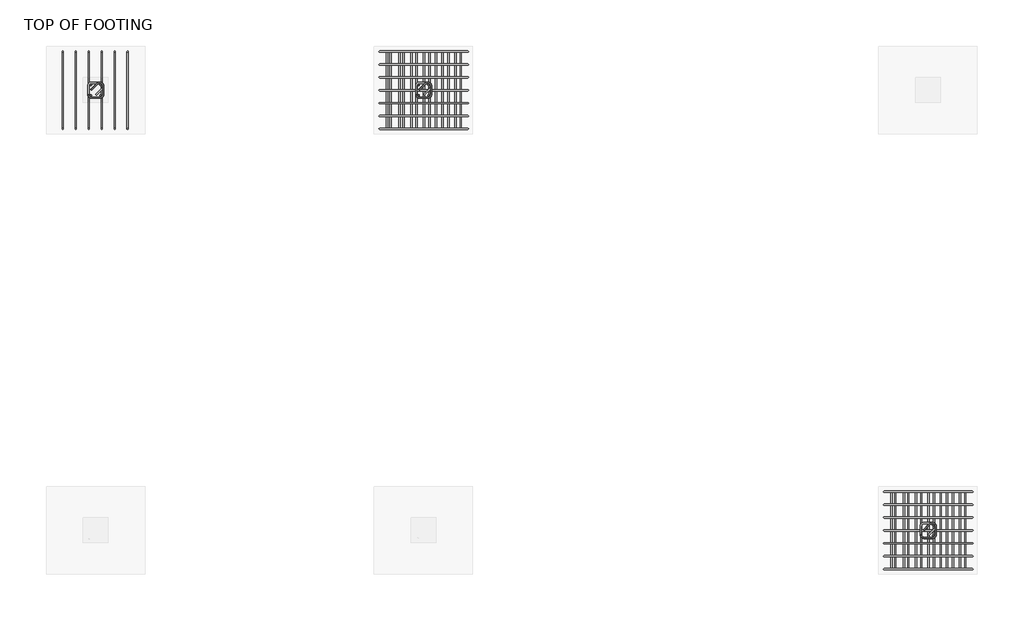
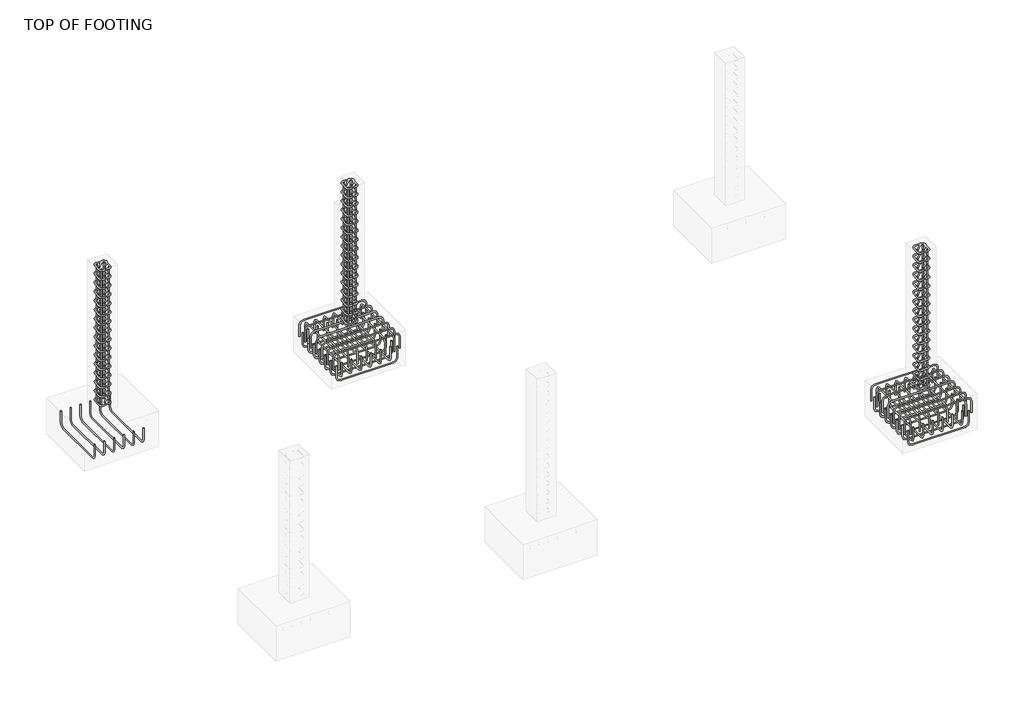
# One storey, part 3 of 6: 17 reinforcing bars.
"""IFC4 building model written with IfcOpenShell, lengths in millimetres."""

from ifc_helpers import new_model, si_unit, point, frame, origin, place, context, project, spatial, polyline, circle_curve, trimmed, segment, composite_curve, source, transform, mapped, element, save
from ifc_brep_helpers import swept_disk

model = new_model("IFC4")

# Units and contexts
model_context = context("Model", 3, world=origin())
ifc_project = project(units=[si_unit("LENGTHUNIT", "METRE", prefix="MILLI")], contexts=[model_context])

# Site, building, storey
site = spatial("IfcSite", under=ifc_project)
building = spatial("IfcBuilding", under=site)
storey = spatial("IfcBuildingStorey", under=building, Name="TOP OF FOOTING", Elevation=-1828.8)

# Reinforcing bars
placement = place(None, origin())
reinforcing_bar_shape = source(origin(), model_context, "Body", "SolidModel", [
    swept_disk(composite_curve([segment(polyline([(-15225.2448384, 120.9474721, -2014.7438142), (-15225.2448384, 120.9474721, -2162.0438142)]), True, "CONTINUOUS"), segment(trimmed(circle_curve(frame((-15225.2448384, 74.5974721, -2162.0438142), z_axis=(-1.0, 0.0, 0.0), x_axis=(0.0, 46.349999999999994, 0.0)), 46.35), [point((-15225.2448384, 120.9474721, -2162.0438142))], [point((-15225.2448384, 74.5974721, -2208.3938142))], True, "CARTESIAN"), True, "CONTINUOUS"), segment(polyline([(-15225.2448384, 74.5974721, -2208.3938142), (-15225.2448384, -540.0025279, -2208.3938142)]), True, "CONTINUOUS"), segment(trimmed(circle_curve(frame((-15225.2448384, -540.0025279, -2162.0438142), z_axis=(-1.0, 0.0, 0.0), x_axis=(0.0, 0.0, -46.350000000000364)), 46.35), [point((-15225.2448384, -540.0025279, -2208.3938142))], [point((-15225.2448384, -586.3525279, -2162.0438142))], True, "CARTESIAN"), True, "CONTINUOUS"), segment(polyline([(-15225.2448384, -586.3525279, -2162.0438142), (-15225.2448384, -586.3525279, -2014.7438142)]), True, "CONTINUOUS")], self_intersect=False), 6.35),
])
element("IfcReinforcingBar", 1, at=placement, inside=storey, context=model_context, shape_type="MappedRepresentation", body=[
    mapped(reinforcing_bar_shape, transform((0.0, 0.0, 0.0), x_axis=(1.0, 0.0, 0.0), y_axis=(0.0, 1.0, 0.0), z_axis=(0.0, 0.0, 1.0))),
    mapped(reinforcing_bar_shape, transform((118.647936, 0.0, 0.0), x_axis=(1.0, 0.0, 0.0), y_axis=(0.0, 1.0, 0.0), z_axis=(0.0, 0.0, 1.0))),
    mapped(reinforcing_bar_shape, transform((237.295872, 0.0, 0.0), x_axis=(1.0, 0.0, 0.0), y_axis=(0.0, 1.0, 0.0), z_axis=(0.0, 0.0, 1.0))),
    mapped(reinforcing_bar_shape, transform((355.943808, 0.0, 0.0), x_axis=(1.0, 0.0, 0.0), y_axis=(0.0, 1.0, 0.0), z_axis=(0.0, 0.0, 1.0))),
    mapped(reinforcing_bar_shape, transform((474.591744, 0.0, 0.0), x_axis=(1.0, 0.0, 0.0), y_axis=(0.0, 1.0, 0.0), z_axis=(0.0, 0.0, 1.0))),
    mapped(reinforcing_bar_shape, transform((593.23968, 0.0, 0.0), x_axis=(1.0, 0.0, 0.0), y_axis=(0.0, 1.0, 0.0), z_axis=(0.0, 0.0, 1.0))),
])
reinforcing_bar_2_shape = source(origin(), model_context, "Body", "SolidModel", [
    swept_disk(composite_curve([segment(polyline([(-11554.9855212, 120.9474721, -2038.8), (-11554.9855212, 120.9474721, -2186.1)]), True, "CONTINUOUS"), segment(trimmed(circle_curve(frame((-11601.3355212, 120.9474721, -2186.1), z_axis=(0.0, 1.0, 0.0), x_axis=(46.350000000000364, 0.0, 0.0)), 46.35), [point((-11554.9855212, 120.9474721, -2186.1))], [point((-11601.3355212, 120.9474721, -2232.45))], True, "CARTESIAN"), True, "CONTINUOUS"), segment(polyline([(-11601.3355212, 120.9474721, -2232.45), (-12244.4761323, 120.9474721, -2232.45)]), True, "CONTINUOUS"), segment(trimmed(circle_curve(frame((-12244.4761323, 120.9474721, -2186.1), z_axis=(0.0, 1.0, 0.0), x_axis=(0.0, 0.0, -46.34999999999991)), 46.35), [point((-12244.4761323, 120.9474721, -2232.45))], [point((-12290.8261323, 120.9474721, -2186.1))], True, "CARTESIAN"), True, "CONTINUOUS"), segment(polyline([(-12290.8261323, 120.9474721, -2186.1), (-12290.8261323, 120.9474721, -2038.8)]), True, "CONTINUOUS")], self_intersect=False), 6.35),
])
element("IfcReinforcingBar", 2, at=placement, inside=storey, context=model_context, shape_type="MappedRepresentation", body=[
    mapped(reinforcing_bar_2_shape, transform((0.0, 0.0, 0.0), x_axis=(1.0, 0.0, 0.0), y_axis=(0.0, 1.0, 0.0), z_axis=(0.0, 0.0, 1.0))),
    mapped(reinforcing_bar_2_shape, transform((0.0, -117.8833333, 0.0), x_axis=(1.0, 0.0, 0.0), y_axis=(0.0, 1.0, 0.0), z_axis=(0.0, 0.0, 1.0))),
    mapped(reinforcing_bar_2_shape, transform((0.0, -235.7666667, 0.0), x_axis=(1.0, 0.0, 0.0), y_axis=(0.0, 1.0, 0.0), z_axis=(0.0, 0.0, 1.0))),
    mapped(reinforcing_bar_2_shape, transform((0.0, -353.65, 0.0), x_axis=(1.0, 0.0, 0.0), y_axis=(0.0, 1.0, 0.0), z_axis=(0.0, 0.0, 1.0))),
    mapped(reinforcing_bar_2_shape, transform((0.0, -471.5333333, 0.0), x_axis=(1.0, 0.0, 0.0), y_axis=(0.0, 1.0, 0.0), z_axis=(0.0, 0.0, 1.0))),
    mapped(reinforcing_bar_2_shape, transform((0.0, -589.4166667, 0.0), x_axis=(1.0, 0.0, 0.0), y_axis=(0.0, 1.0, 0.0), z_axis=(0.0, 0.0, 1.0))),
    mapped(reinforcing_bar_2_shape, transform((0.0, -707.3, 0.0), x_axis=(1.0, 0.0, 0.0), y_axis=(0.0, 1.0, 0.0), z_axis=(0.0, 0.0, 1.0))),
])
reinforcing_bar_3_shape = source(origin(), model_context, "Body", "SolidModel", [
    swept_disk(composite_curve([segment(polyline([(-12330.2056799, 120.9474721, -2070.9463075), (-12330.2056799, 120.9474721, -1923.6463075)]), True, "CONTINUOUS"), segment(trimmed(circle_curve(frame((-12283.8556799, 120.9474721, -1923.6463075), z_axis=(0.0, 1.0, 0.0), x_axis=(-46.350000000000364, 0.0, 0.0)), 46.35), [point((-12330.2056799, 120.9474721, -1923.6463075))], [point((-12283.8556799, 120.9474721, -1877.2963075))], True, "CARTESIAN"), True, "CONTINUOUS"), segment(polyline([(-12283.8556799, 120.9474721, -1877.2963075), (-11569.2556799, 120.9474721, -1877.2963075)]), True, "CONTINUOUS"), segment(trimmed(circle_curve(frame((-11569.2556799, 120.9474721, -1923.6463075), z_axis=(0.0, 1.0, 0.0), x_axis=(0.0, 0.0, 46.34999999999991)), 46.35), [point((-11569.2556799, 120.9474721, -1877.2963075))], [point((-11522.9056799, 120.9474721, -1923.6463075))], True, "CARTESIAN"), True, "CONTINUOUS"), segment(polyline([(-11522.9056799, 120.9474721, -1923.6463075), (-11522.9056799, 120.9474721, -2070.9463075)]), True, "CONTINUOUS")], self_intersect=False), 6.35),
])
element("IfcReinforcingBar", 3, at=placement, inside=storey, context=model_context, shape_type="MappedRepresentation", body=[
    mapped(reinforcing_bar_3_shape, transform((0.0, 0.0, 0.0), x_axis=(1.0, 0.0, 0.0), y_axis=(0.0, 1.0, 0.0), z_axis=(0.0, 0.0, 1.0))),
    mapped(reinforcing_bar_3_shape, transform((0.0, -117.8833333, 0.0), x_axis=(1.0, 0.0, 0.0), y_axis=(0.0, 1.0, 0.0), z_axis=(0.0, 0.0, 1.0))),
    mapped(reinforcing_bar_3_shape, transform((0.0, -235.7666667, 0.0), x_axis=(1.0, 0.0, 0.0), y_axis=(0.0, 1.0, 0.0), z_axis=(0.0, 0.0, 1.0))),
    mapped(reinforcing_bar_3_shape, transform((0.0, -353.65, 0.0), x_axis=(1.0, 0.0, 0.0), y_axis=(0.0, 1.0, 0.0), z_axis=(0.0, 0.0, 1.0))),
    mapped(reinforcing_bar_3_shape, transform((0.0, -471.5333333, 0.0), x_axis=(1.0, 0.0, 0.0), y_axis=(0.0, 1.0, 0.0), z_axis=(0.0, 0.0, 1.0))),
    mapped(reinforcing_bar_3_shape, transform((0.0, -589.4166667, 0.0), x_axis=(1.0, 0.0, 0.0), y_axis=(0.0, 1.0, 0.0), z_axis=(0.0, 0.0, 1.0))),
    mapped(reinforcing_bar_3_shape, transform((0.0, -707.3, 0.0), x_axis=(1.0, 0.0, 0.0), y_axis=(0.0, 1.0, 0.0), z_axis=(0.0, 0.0, 1.0))),
])
reinforcing_bar_4_shape = source(origin(), model_context, "Body", "SolidModel", [
    swept_disk(composite_curve([segment(polyline([(-11588.0545962, 120.9474721, -2094.0228735), (-11588.0545962, 120.9474721, -1946.7228735)]), True, "CONTINUOUS"), segment(trimmed(circle_curve(frame((-11588.0545962, 74.5974721, -1946.7228735), z_axis=(1.0, 0.0, 0.0), x_axis=(0.0, 46.349999999999994, 0.0)), 46.35), [point((-11588.0545962, 120.9474721, -1946.7228735))], [point((-11588.0545962, 74.5974721, -1900.3728735))], True, "CARTESIAN"), True, "CONTINUOUS"), segment(polyline([(-11588.0545962, 74.5974721, -1900.3728735), (-11588.0545962, -540.0025279, -1900.3728735)]), True, "CONTINUOUS"), segment(trimmed(circle_curve(frame((-11588.0545962, -540.0025279, -1946.7228735), z_axis=(1.0, 0.0, 0.0), x_axis=(0.0, 0.0, 46.350000000000136)), 46.35), [point((-11588.0545962, -540.0025279, -1900.3728735))], [point((-11588.0545962, -586.3525279, -1946.7228735))], True, "CARTESIAN"), True, "CONTINUOUS"), segment(polyline([(-11588.0545962, -586.3525279, -1946.7228735), (-11588.0545962, -586.3525279, -2094.0228735)]), True, "CONTINUOUS")], self_intersect=False), 6.35),
])
element("IfcReinforcingBar", 4, at=placement, inside=storey, context=model_context, shape_type="MappedRepresentation", body=[
    mapped(reinforcing_bar_4_shape, transform((0.0, 0.0, 0.0), x_axis=(1.0, 0.0, 0.0), y_axis=(0.0, 1.0, 0.0), z_axis=(0.0, 0.0, 1.0))),
    mapped(reinforcing_bar_4_shape, transform((-112.124631, 0.0, 0.0), x_axis=(1.0, 0.0, 0.0), y_axis=(0.0, 1.0, 0.0), z_axis=(0.0, 0.0, 1.0))),
    mapped(reinforcing_bar_4_shape, transform((-224.2492621, 0.0, 0.0), x_axis=(1.0, 0.0, 0.0), y_axis=(0.0, 1.0, 0.0), z_axis=(0.0, 0.0, 1.0))),
    mapped(reinforcing_bar_4_shape, transform((-336.3738931, 0.0, 0.0), x_axis=(1.0, 0.0, 0.0), y_axis=(0.0, 1.0, 0.0), z_axis=(0.0, 0.0, 1.0))),
    mapped(reinforcing_bar_4_shape, transform((-448.4985241, 0.0, 0.0), x_axis=(1.0, 0.0, 0.0), y_axis=(0.0, 1.0, 0.0), z_axis=(0.0, 0.0, 1.0))),
    mapped(reinforcing_bar_4_shape, transform((-560.6231552, 0.0, 0.0), x_axis=(1.0, 0.0, 0.0), y_axis=(0.0, 1.0, 0.0), z_axis=(0.0, 0.0, 1.0))),
    mapped(reinforcing_bar_4_shape, transform((-672.7477862, 0.0, 0.0), x_axis=(1.0, 0.0, 0.0), y_axis=(0.0, 1.0, 0.0), z_axis=(0.0, 0.0, 1.0))),
])
reinforcing_bar_5_shape = source(origin(), model_context, "Body", "SolidModel", [
    swept_disk(composite_curve([segment(polyline([(-12228.0448384, 120.9474721, -2014.7438142), (-12228.0448384, 120.9474721, -2162.0438142)]), True, "CONTINUOUS"), segment(trimmed(circle_curve(frame((-12228.0448384, 74.5974721, -2162.0438142), z_axis=(-1.0, 0.0, 0.0), x_axis=(0.0, 46.349999999999994, 0.0)), 46.35), [point((-12228.0448384, 120.9474721, -2162.0438142))], [point((-12228.0448384, 74.5974721, -2208.3938142))], True, "CARTESIAN"), True, "CONTINUOUS"), segment(polyline([(-12228.0448384, 74.5974721, -2208.3938142), (-12228.0448384, -540.0025279, -2208.3938142)]), True, "CONTINUOUS"), segment(trimmed(circle_curve(frame((-12228.0448384, -540.0025279, -2162.0438142), z_axis=(-1.0, 0.0, 0.0), x_axis=(0.0, 0.0, -46.350000000000364)), 46.35), [point((-12228.0448384, -540.0025279, -2208.3938142))], [point((-12228.0448384, -586.3525279, -2162.0438142))], True, "CARTESIAN"), True, "CONTINUOUS"), segment(polyline([(-12228.0448384, -586.3525279, -2162.0438142), (-12228.0448384, -586.3525279, -2014.7438142)]), True, "CONTINUOUS")], self_intersect=False), 6.35),
])
element("IfcReinforcingBar", 5, at=placement, inside=storey, context=model_context, shape_type="MappedRepresentation", body=[
    mapped(reinforcing_bar_5_shape, transform((0.0, 0.0, 0.0), x_axis=(1.0, 0.0, 0.0), y_axis=(0.0, 1.0, 0.0), z_axis=(0.0, 0.0, 1.0))),
    mapped(reinforcing_bar_5_shape, transform((118.647936, 0.0, 0.0), x_axis=(1.0, 0.0, 0.0), y_axis=(0.0, 1.0, 0.0), z_axis=(0.0, 0.0, 1.0))),
    mapped(reinforcing_bar_5_shape, transform((237.295872, 0.0, 0.0), x_axis=(1.0, 0.0, 0.0), y_axis=(0.0, 1.0, 0.0), z_axis=(0.0, 0.0, 1.0))),
    mapped(reinforcing_bar_5_shape, transform((355.943808, 0.0, 0.0), x_axis=(1.0, 0.0, 0.0), y_axis=(0.0, 1.0, 0.0), z_axis=(0.0, 0.0, 1.0))),
    mapped(reinforcing_bar_5_shape, transform((474.591744, 0.0, 0.0), x_axis=(1.0, 0.0, 0.0), y_axis=(0.0, 1.0, 0.0), z_axis=(0.0, 0.0, 1.0))),
    mapped(reinforcing_bar_5_shape, transform((593.23968, 0.0, 0.0), x_axis=(1.0, 0.0, 0.0), y_axis=(0.0, 1.0, 0.0), z_axis=(0.0, 0.0, 1.0))),
])
reinforcing_bar_6_shape = source(origin(), model_context, "Body", "SolidModel", [
    swept_disk(composite_curve([segment(polyline([(-6942.8971795, -3906.2483349, -2038.8), (-6942.8971795, -3906.2483349, -2186.1)]), True, "CONTINUOUS"), segment(trimmed(circle_curve(frame((-6989.2471795, -3906.2483349, -2186.1), z_axis=(0.0, 1.0, 0.0), x_axis=(46.350000000000364, 0.0, 0.0)), 46.35), [point((-6942.8971795, -3906.2483349, -2186.1))], [point((-6989.2471795, -3906.2483349, -2232.45))], True, "CARTESIAN"), True, "CONTINUOUS"), segment(polyline([(-6989.2471795, -3906.2483349, -2232.45), (-7632.3877906, -3906.2483349, -2232.45)]), True, "CONTINUOUS"), segment(trimmed(circle_curve(frame((-7632.3877906, -3906.2483349, -2186.1), z_axis=(0.0, 1.0, 0.0), x_axis=(0.0, 0.0, -46.34999999999991)), 46.35), [point((-7632.3877906, -3906.2483349, -2232.45))], [point((-7678.7377906, -3906.2483349, -2186.1))], True, "CARTESIAN"), True, "CONTINUOUS"), segment(polyline([(-7678.7377906, -3906.2483349, -2186.1), (-7678.7377906, -3906.2483349, -2038.8)]), True, "CONTINUOUS")], self_intersect=False), 6.35),
])
element("IfcReinforcingBar", 6, at=placement, inside=storey, context=model_context, shape_type="MappedRepresentation", body=[
    mapped(reinforcing_bar_6_shape, transform((0.0, 0.0, 0.0), x_axis=(1.0, 0.0, 0.0), y_axis=(0.0, 1.0, 0.0), z_axis=(0.0, 0.0, 1.0))),
    mapped(reinforcing_bar_6_shape, transform((0.0, -117.8833333, 0.0), x_axis=(1.0, 0.0, 0.0), y_axis=(0.0, 1.0, 0.0), z_axis=(0.0, 0.0, 1.0))),
    mapped(reinforcing_bar_6_shape, transform((0.0, -235.7666667, 0.0), x_axis=(1.0, 0.0, 0.0), y_axis=(0.0, 1.0, 0.0), z_axis=(0.0, 0.0, 1.0))),
    mapped(reinforcing_bar_6_shape, transform((0.0, -353.65, 0.0), x_axis=(1.0, 0.0, 0.0), y_axis=(0.0, 1.0, 0.0), z_axis=(0.0, 0.0, 1.0))),
    mapped(reinforcing_bar_6_shape, transform((0.0, -471.5333333, 0.0), x_axis=(1.0, 0.0, 0.0), y_axis=(0.0, 1.0, 0.0), z_axis=(0.0, 0.0, 1.0))),
    mapped(reinforcing_bar_6_shape, transform((0.0, -589.4166667, 0.0), x_axis=(1.0, 0.0, 0.0), y_axis=(0.0, 1.0, 0.0), z_axis=(0.0, 0.0, 1.0))),
    mapped(reinforcing_bar_6_shape, transform((0.0, -707.3, 0.0), x_axis=(1.0, 0.0, 0.0), y_axis=(0.0, 1.0, 0.0), z_axis=(0.0, 0.0, 1.0))),
])
reinforcing_bar_7_shape = source(origin(), model_context, "Body", "SolidModel", [
    swept_disk(composite_curve([segment(polyline([(-7718.1173382, -3906.2483349, -2070.9463075), (-7718.1173382, -3906.2483349, -1923.6463075)]), True, "CONTINUOUS"), segment(trimmed(circle_curve(frame((-7671.7673382, -3906.2483349, -1923.6463075), z_axis=(0.0, 1.0, 0.0), x_axis=(-46.349999999999454, 0.0, 0.0)), 46.35), [point((-7718.1173382, -3906.2483349, -1923.6463075))], [point((-7671.7673382, -3906.2483349, -1877.2963075))], True, "CARTESIAN"), True, "CONTINUOUS"), segment(polyline([(-7671.7673382, -3906.2483349, -1877.2963075), (-6957.1673382, -3906.2483349, -1877.2963075)]), True, "CONTINUOUS"), segment(trimmed(circle_curve(frame((-6957.1673382, -3906.2483349, -1923.6463075), z_axis=(0.0, 1.0, 0.0), x_axis=(0.0, 0.0, 46.34999999999991)), 46.35), [point((-6957.1673382, -3906.2483349, -1877.2963075))], [point((-6910.8173382, -3906.2483349, -1923.6463075))], True, "CARTESIAN"), True, "CONTINUOUS"), segment(polyline([(-6910.8173382, -3906.2483349, -1923.6463075), (-6910.8173382, -3906.2483349, -2070.9463075)]), True, "CONTINUOUS")], self_intersect=False), 6.35),
])
element("IfcReinforcingBar", 7, at=placement, inside=storey, context=model_context, shape_type="MappedRepresentation", body=[
    mapped(reinforcing_bar_7_shape, transform((0.0, 0.0, 0.0), x_axis=(1.0, 0.0, 0.0), y_axis=(0.0, 1.0, 0.0), z_axis=(0.0, 0.0, 1.0))),
    mapped(reinforcing_bar_7_shape, transform((0.0, -117.8833333, 0.0), x_axis=(1.0, 0.0, 0.0), y_axis=(0.0, 1.0, 0.0), z_axis=(0.0, 0.0, 1.0))),
    mapped(reinforcing_bar_7_shape, transform((0.0, -235.7666667, 0.0), x_axis=(1.0, 0.0, 0.0), y_axis=(0.0, 1.0, 0.0), z_axis=(0.0, 0.0, 1.0))),
    mapped(reinforcing_bar_7_shape, transform((0.0, -353.65, 0.0), x_axis=(1.0, 0.0, 0.0), y_axis=(0.0, 1.0, 0.0), z_axis=(0.0, 0.0, 1.0))),
    mapped(reinforcing_bar_7_shape, transform((0.0, -471.5333333, 0.0), x_axis=(1.0, 0.0, 0.0), y_axis=(0.0, 1.0, 0.0), z_axis=(0.0, 0.0, 1.0))),
    mapped(reinforcing_bar_7_shape, transform((0.0, -589.4166667, 0.0), x_axis=(1.0, 0.0, 0.0), y_axis=(0.0, 1.0, 0.0), z_axis=(0.0, 0.0, 1.0))),
    mapped(reinforcing_bar_7_shape, transform((0.0, -707.3, 0.0), x_axis=(1.0, 0.0, 0.0), y_axis=(0.0, 1.0, 0.0), z_axis=(0.0, 0.0, 1.0))),
])
reinforcing_bar_8_shape = source(origin(), model_context, "Body", "SolidModel", [
    swept_disk(composite_curve([segment(polyline([(-6975.9662545, -3906.2483349, -2094.0228735), (-6975.9662545, -3906.2483349, -1946.7228735)]), True, "CONTINUOUS"), segment(trimmed(circle_curve(frame((-6975.9662545, -3952.5983349, -1946.7228735), z_axis=(1.0, 0.0, 0.0), x_axis=(0.0, 46.34999999999991, 0.0)), 46.35), [point((-6975.9662545, -3906.2483349, -1946.7228735))], [point((-6975.9662545, -3952.5983349, -1900.3728735))], True, "CARTESIAN"), True, "CONTINUOUS"), segment(polyline([(-6975.9662545, -3952.5983349, -1900.3728735), (-6975.9662545, -4567.1983349, -1900.3728735)]), True, "CONTINUOUS"), segment(trimmed(circle_curve(frame((-6975.9662545, -4567.1983349, -1946.7228735), z_axis=(1.0, 0.0, 0.0), x_axis=(0.0, 0.0, 46.350000000000136)), 46.35), [point((-6975.9662545, -4567.1983349, -1900.3728735))], [point((-6975.9662545, -4613.5483349, -1946.7228735))], True, "CARTESIAN"), True, "CONTINUOUS"), segment(polyline([(-6975.9662545, -4613.5483349, -1946.7228735), (-6975.9662545, -4613.5483349, -2094.0228735)]), True, "CONTINUOUS")], self_intersect=False), 6.35),
])
element("IfcReinforcingBar", 8, at=placement, inside=storey, context=model_context, shape_type="MappedRepresentation", body=[
    mapped(reinforcing_bar_8_shape, transform((0.0, 0.0, 0.0), x_axis=(1.0, 0.0, 0.0), y_axis=(0.0, 1.0, 0.0), z_axis=(0.0, 0.0, 1.0))),
    mapped(reinforcing_bar_8_shape, transform((-112.124631, 0.0, 0.0), x_axis=(1.0, 0.0, 0.0), y_axis=(0.0, 1.0, 0.0), z_axis=(0.0, 0.0, 1.0))),
    mapped(reinforcing_bar_8_shape, transform((-224.2492621, 0.0, 0.0), x_axis=(1.0, 0.0, 0.0), y_axis=(0.0, 1.0, 0.0), z_axis=(0.0, 0.0, 1.0))),
    mapped(reinforcing_bar_8_shape, transform((-336.3738931, 0.0, 0.0), x_axis=(1.0, 0.0, 0.0), y_axis=(0.0, 1.0, 0.0), z_axis=(0.0, 0.0, 1.0))),
    mapped(reinforcing_bar_8_shape, transform((-448.4985241, 0.0, 0.0), x_axis=(1.0, 0.0, 0.0), y_axis=(0.0, 1.0, 0.0), z_axis=(0.0, 0.0, 1.0))),
    mapped(reinforcing_bar_8_shape, transform((-560.6231552, 0.0, 0.0), x_axis=(1.0, 0.0, 0.0), y_axis=(0.0, 1.0, 0.0), z_axis=(0.0, 0.0, 1.0))),
    mapped(reinforcing_bar_8_shape, transform((-672.7477862, 0.0, 0.0), x_axis=(1.0, 0.0, 0.0), y_axis=(0.0, 1.0, 0.0), z_axis=(0.0, 0.0, 1.0))),
])
reinforcing_bar_9_shape = source(origin(), model_context, "Body", "SolidModel", [
    swept_disk(composite_curve([segment(polyline([(-7615.9564967, -3906.2483349, -2014.7438142), (-7615.9564967, -3906.2483349, -2162.0438142)]), True, "CONTINUOUS"), segment(trimmed(circle_curve(frame((-7615.9564967, -3952.5983349, -2162.0438142), z_axis=(-1.0, 0.0, 0.0), x_axis=(0.0, 46.34999999999991, 0.0)), 46.35), [point((-7615.9564967, -3906.2483349, -2162.0438142))], [point((-7615.9564967, -3952.5983349, -2208.3938142))], True, "CARTESIAN"), True, "CONTINUOUS"), segment(polyline([(-7615.9564967, -3952.5983349, -2208.3938142), (-7615.9564967, -4567.1983349, -2208.3938142)]), True, "CONTINUOUS"), segment(trimmed(circle_curve(frame((-7615.9564967, -4567.1983349, -2162.0438142), z_axis=(-1.0, 0.0, 0.0), x_axis=(0.0, 0.0, -46.350000000000364)), 46.35), [point((-7615.9564967, -4567.1983349, -2208.3938142))], [point((-7615.9564967, -4613.5483349, -2162.0438142))], True, "CARTESIAN"), True, "CONTINUOUS"), segment(polyline([(-7615.9564967, -4613.5483349, -2162.0438142), (-7615.9564967, -4613.5483349, -2014.7438142)]), True, "CONTINUOUS")], self_intersect=False), 6.35),
])
element("IfcReinforcingBar", 9, at=placement, inside=storey, context=model_context, shape_type="MappedRepresentation", body=[
    mapped(reinforcing_bar_9_shape, transform((0.0, 0.0, 0.0), x_axis=(1.0, 0.0, 0.0), y_axis=(0.0, 1.0, 0.0), z_axis=(0.0, 0.0, 1.0))),
    mapped(reinforcing_bar_9_shape, transform((118.647936, 0.0, 0.0), x_axis=(1.0, 0.0, 0.0), y_axis=(0.0, 1.0, 0.0), z_axis=(0.0, 0.0, 1.0))),
    mapped(reinforcing_bar_9_shape, transform((237.295872, 0.0, 0.0), x_axis=(1.0, 0.0, 0.0), y_axis=(0.0, 1.0, 0.0), z_axis=(0.0, 0.0, 1.0))),
    mapped(reinforcing_bar_9_shape, transform((355.943808, 0.0, 0.0), x_axis=(1.0, 0.0, 0.0), y_axis=(0.0, 1.0, 0.0), z_axis=(0.0, 0.0, 1.0))),
    mapped(reinforcing_bar_9_shape, transform((474.591744, 0.0, 0.0), x_axis=(1.0, 0.0, 0.0), y_axis=(0.0, 1.0, 0.0), z_axis=(0.0, 0.0, 1.0))),
    mapped(reinforcing_bar_9_shape, transform((593.23968, 0.0, 0.0), x_axis=(1.0, 0.0, 0.0), y_axis=(0.0, 1.0, 0.0), z_axis=(0.0, 0.0, 1.0))),
])
reinforcing_bar_10_shape = source(origin(), model_context, "Body", "SolidModel", [
    swept_disk(composite_curve([segment(polyline([(-7269.7123519, -4211.1006392, -40.0), (-7269.7123519, -4211.1006392, -1788.8)]), True, "CONTINUOUS")], self_intersect=False), 6.35),
])
element("IfcReinforcingBar", 10, at=placement, inside=storey, context=model_context, shape_type="MappedRepresentation", body=[
    mapped(reinforcing_bar_10_shape, transform((0.0, 0.0, 0.0), x_axis=(1.0, 0.0, 0.0), y_axis=(0.0, 1.0, 0.0), z_axis=(0.0, 0.0, 1.0))),
    mapped(reinforcing_bar_10_shape, transform((0.0, -96.9916148, 0.0), x_axis=(1.0, 0.0, 0.0), y_axis=(0.0, 1.0, 0.0), z_axis=(0.0, 0.0, 1.0))),
])
reinforcing_bar_11_shape = source(origin(), model_context, "Body", "SolidModel", [
    swept_disk(composite_curve([segment(polyline([(-7355.7786987, -4256.8741003, -46.35), (-7300.0351358, -4201.1305373, -46.35)]), True, "CONTINUOUS"), segment(trimmed(circle_curve(frame((-7277.8673382, -4223.2983349, -46.35), z_axis=(0.0, 0.0, -1.0), x_axis=(-22.167797600000085, 22.167797600000085, 0.0)), 31.35), [point((-7300.0351358, -4201.1305373, -46.35))], [point((-7246.5173382, -4223.2983349, -46.35))], True, "CARTESIAN"), True, "CONTINUOUS"), segment(polyline([(-7246.5173382, -4223.2983349, -46.35), (-7246.5173382, -4296.4983349, -46.35)]), True, "CONTINUOUS"), segment(trimmed(circle_curve(frame((-7277.8673382, -4296.4983349, -46.35), z_axis=(0.0, 0.0, -1.0), x_axis=(31.349999999999454, 0.0, 0.0)), 31.35), [point((-7246.5173382, -4296.4983349, -46.35))], [point((-7277.8673382, -4327.8483349, -46.35))], True, "CARTESIAN"), True, "CONTINUOUS"), segment(polyline([(-7277.8673382, -4327.8483349, -46.35), (-7351.0673382, -4327.8483349, -46.35)]), True, "CONTINUOUS"), segment(trimmed(circle_curve(frame((-7351.0673382, -4296.6343361, -43.4330185), z_axis=(0.0, 0.09304566152621355, -0.9956618426308951), x_axis=(0.0, -31.2139987999999, -2.9169814999999986)), 31.35), [point((-7351.0673382, -4327.8483349, -46.35))], [point((-7382.4173382, -4296.6343361, -43.4330185))], True, "CARTESIAN"), True, "CONTINUOUS"), segment(polyline([(-7382.4173382, -4296.6343361, -43.4330185), (-7382.4173382, -4223.1623337, -36.5669815)]), True, "CONTINUOUS"), segment(trimmed(circle_curve(frame((-7351.0673382, -4223.1623337, -36.5669815), z_axis=(0.0, 0.09304566152621355, -0.9956618426308951), x_axis=(-31.349999999999454, 0.0, 0.0)), 31.35), [point((-7382.4173382, -4223.1623337, -36.5669815))], [point((-7351.0673382, -4191.9483349, -33.65))], True, "CARTESIAN"), True, "CONTINUOUS"), segment(polyline([(-7351.0673382, -4191.9483349, -33.65), (-7277.8673382, -4191.9483349, -33.65)]), True, "CONTINUOUS"), segment(trimmed(circle_curve(frame((-7277.8673382, -4223.2983349, -33.65), z_axis=(0.0, 0.0, -1.0), x_axis=(0.0, 31.349999999999454, 0.0)), 31.35), [point((-7277.8673382, -4191.9483349, -33.65))], [point((-7255.6995406, -4245.4661325, -33.65))], True, "CARTESIAN"), True, "CONTINUOUS"), segment(polyline([(-7255.6995406, -4245.4661325, -33.65), (-7311.4431035, -4301.2096954, -33.65)]), True, "CONTINUOUS")], self_intersect=False), 6.35),
])
element("IfcReinforcingBar", 11, at=placement, inside=storey, context=model_context, shape_type="MappedRepresentation", body=[
    mapped(reinforcing_bar_11_shape, transform((0.0, 0.0, 0.0), x_axis=(1.0, 0.0, 0.0), y_axis=(0.0, 1.0, 0.0), z_axis=(0.0, 0.0, 1.0))),
    mapped(reinforcing_bar_11_shape, transform((0.0, 0.0, -115.74), x_axis=(1.0, 0.0, 0.0), y_axis=(0.0, 1.0, 0.0), z_axis=(0.0, 0.0, 1.0))),
    mapped(reinforcing_bar_11_shape, transform((0.0, 0.0, -231.48), x_axis=(1.0, 0.0, 0.0), y_axis=(0.0, 1.0, 0.0), z_axis=(0.0, 0.0, 1.0))),
    mapped(reinforcing_bar_11_shape, transform((0.0, 0.0, -347.22), x_axis=(1.0, 0.0, 0.0), y_axis=(0.0, 1.0, 0.0), z_axis=(0.0, 0.0, 1.0))),
    mapped(reinforcing_bar_11_shape, transform((0.0, 0.0, -462.96), x_axis=(1.0, 0.0, 0.0), y_axis=(0.0, 1.0, 0.0), z_axis=(0.0, 0.0, 1.0))),
    mapped(reinforcing_bar_11_shape, transform((0.0, 0.0, -578.7), x_axis=(1.0, 0.0, 0.0), y_axis=(0.0, 1.0, 0.0), z_axis=(0.0, 0.0, 1.0))),
    mapped(reinforcing_bar_11_shape, transform((0.0, 0.0, -694.44), x_axis=(1.0, 0.0, 0.0), y_axis=(0.0, 1.0, 0.0), z_axis=(0.0, 0.0, 1.0))),
    mapped(reinforcing_bar_11_shape, transform((0.0, 0.0, -810.18), x_axis=(1.0, 0.0, 0.0), y_axis=(0.0, 1.0, 0.0), z_axis=(0.0, 0.0, 1.0))),
    mapped(reinforcing_bar_11_shape, transform((0.0, 0.0, -925.92), x_axis=(1.0, 0.0, 0.0), y_axis=(0.0, 1.0, 0.0), z_axis=(0.0, 0.0, 1.0))),
    mapped(reinforcing_bar_11_shape, transform((0.0, 0.0, -1041.66), x_axis=(1.0, 0.0, 0.0), y_axis=(0.0, 1.0, 0.0), z_axis=(0.0, 0.0, 1.0))),
    mapped(reinforcing_bar_11_shape, transform((0.0, 0.0, -1157.4), x_axis=(1.0, 0.0, 0.0), y_axis=(0.0, 1.0, 0.0), z_axis=(0.0, 0.0, 1.0))),
    mapped(reinforcing_bar_11_shape, transform((0.0, 0.0, -1273.14), x_axis=(1.0, 0.0, 0.0), y_axis=(0.0, 1.0, 0.0), z_axis=(0.0, 0.0, 1.0))),
    mapped(reinforcing_bar_11_shape, transform((0.0, 0.0, -1388.88), x_axis=(1.0, 0.0, 0.0), y_axis=(0.0, 1.0, 0.0), z_axis=(0.0, 0.0, 1.0))),
    mapped(reinforcing_bar_11_shape, transform((0.0, 0.0, -1504.62), x_axis=(1.0, 0.0, 0.0), y_axis=(0.0, 1.0, 0.0), z_axis=(0.0, 0.0, 1.0))),
    mapped(reinforcing_bar_11_shape, transform((0.0, 0.0, -1620.36), x_axis=(1.0, 0.0, 0.0), y_axis=(0.0, 1.0, 0.0), z_axis=(0.0, 0.0, 1.0))),
    mapped(reinforcing_bar_11_shape, transform((0.0, 0.0, -1736.1), x_axis=(1.0, 0.0, 0.0), y_axis=(0.0, 1.0, 0.0), z_axis=(0.0, 0.0, 1.0))),
])
reinforcing_bar_12_shape = source(origin(), model_context, "Body", "SolidModel", [
    swept_disk(composite_curve([segment(polyline([(-14879.0006936, -183.9048321, -40.0), (-14879.0006936, -183.9048321, -1788.8)]), True, "CONTINUOUS")], self_intersect=False), 6.35),
])
element("IfcReinforcingBar", 12, at=placement, inside=storey, context=model_context, shape_type="MappedRepresentation", body=[
    mapped(reinforcing_bar_12_shape, transform((0.0, 0.0, 0.0), x_axis=(1.0, 0.0, 0.0), y_axis=(0.0, 1.0, 0.0), z_axis=(0.0, 0.0, 1.0))),
    mapped(reinforcing_bar_12_shape, transform((0.0, -96.9916148, 0.0), x_axis=(1.0, 0.0, 0.0), y_axis=(0.0, 1.0, 0.0), z_axis=(0.0, 0.0, 1.0))),
])
reinforcing_bar_13_shape = source(origin(), model_context, "Body", "SolidModel", [
    swept_disk(composite_curve([segment(polyline([(-14965.0670404, -229.6782932, -46.35), (-14909.3234775, -173.9347303, -46.35)]), True, "CONTINUOUS"), segment(trimmed(circle_curve(frame((-14887.1556799, -196.1025279, -46.35), z_axis=(0.0, 0.0, -1.0), x_axis=(-22.167797599999176, 22.1677976, 0.0)), 31.35), [point((-14909.3234775, -173.9347303, -46.35))], [point((-14855.8056799, -196.1025279, -46.35))], True, "CARTESIAN"), True, "CONTINUOUS"), segment(polyline([(-14855.8056799, -196.1025279, -46.35), (-14855.8056799, -269.3025279, -46.35)]), True, "CONTINUOUS"), segment(trimmed(circle_curve(frame((-14887.1556799, -269.3025279, -46.35), z_axis=(0.0, 0.0, -1.0), x_axis=(31.350000000000364, 0.0, 0.0)), 31.35), [point((-14855.8056799, -269.3025279, -46.35))], [point((-14887.1556799, -300.6525279, -46.35))], True, "CARTESIAN"), True, "CONTINUOUS"), segment(polyline([(-14887.1556799, -300.6525279, -46.35), (-14960.3556799, -300.6525279, -46.35)]), True, "CONTINUOUS"), segment(trimmed(circle_curve(frame((-14960.3556799, -269.4385291, -43.4330185), z_axis=(0.0, 0.09304566152621355, -0.9956618426308951), x_axis=(0.0, -31.213998800000013, -2.9169814999999986)), 31.35), [point((-14960.3556799, -300.6525279, -46.35))], [point((-14991.7056799, -269.4385291, -43.4330185))], True, "CARTESIAN"), True, "CONTINUOUS"), segment(polyline([(-14991.7056799, -269.4385291, -43.4330185), (-14991.7056799, -195.9665266, -36.5669815)]), True, "CONTINUOUS"), segment(trimmed(circle_curve(frame((-14960.3556799, -195.9665266, -36.5669815), z_axis=(0.0, 0.09304566152621355, -0.9956618426308951), x_axis=(-31.350000000000364, 0.0, 0.0)), 31.35), [point((-14991.7056799, -195.9665266, -36.5669815))], [point((-14960.3556799, -164.7525279, -33.65))], True, "CARTESIAN"), True, "CONTINUOUS"), segment(polyline([(-14960.3556799, -164.7525279, -33.65), (-14887.1556799, -164.7525279, -33.65)]), True, "CONTINUOUS"), segment(trimmed(circle_curve(frame((-14887.1556799, -196.1025279, -33.65), z_axis=(0.0, 0.0, -1.0), x_axis=(0.0, 31.350000000000023, 0.0)), 31.35), [point((-14887.1556799, -164.7525279, -33.65))], [point((-14864.9878823, -218.2703255, -33.65))], True, "CARTESIAN"), True, "CONTINUOUS"), segment(polyline([(-14864.9878823, -218.2703255, -33.65), (-14920.7314452, -274.0138884, -33.65)]), True, "CONTINUOUS")], self_intersect=False), 6.35),
])
element("IfcReinforcingBar", 13, at=placement, inside=storey, context=model_context, shape_type="MappedRepresentation", body=[
    mapped(reinforcing_bar_13_shape, transform((0.0, 0.0, 0.0), x_axis=(1.0, 0.0, 0.0), y_axis=(0.0, 1.0, 0.0), z_axis=(0.0, 0.0, 1.0))),
    mapped(reinforcing_bar_13_shape, transform((0.0, 0.0, -115.74), x_axis=(1.0, 0.0, 0.0), y_axis=(0.0, 1.0, 0.0), z_axis=(0.0, 0.0, 1.0))),
    mapped(reinforcing_bar_13_shape, transform((0.0, 0.0, -231.48), x_axis=(1.0, 0.0, 0.0), y_axis=(0.0, 1.0, 0.0), z_axis=(0.0, 0.0, 1.0))),
    mapped(reinforcing_bar_13_shape, transform((0.0, 0.0, -347.22), x_axis=(1.0, 0.0, 0.0), y_axis=(0.0, 1.0, 0.0), z_axis=(0.0, 0.0, 1.0))),
    mapped(reinforcing_bar_13_shape, transform((0.0, 0.0, -462.96), x_axis=(1.0, 0.0, 0.0), y_axis=(0.0, 1.0, 0.0), z_axis=(0.0, 0.0, 1.0))),
    mapped(reinforcing_bar_13_shape, transform((0.0, 0.0, -578.7), x_axis=(1.0, 0.0, 0.0), y_axis=(0.0, 1.0, 0.0), z_axis=(0.0, 0.0, 1.0))),
    mapped(reinforcing_bar_13_shape, transform((0.0, 0.0, -694.44), x_axis=(1.0, 0.0, 0.0), y_axis=(0.0, 1.0, 0.0), z_axis=(0.0, 0.0, 1.0))),
    mapped(reinforcing_bar_13_shape, transform((0.0, 0.0, -810.18), x_axis=(1.0, 0.0, 0.0), y_axis=(0.0, 1.0, 0.0), z_axis=(0.0, 0.0, 1.0))),
    mapped(reinforcing_bar_13_shape, transform((0.0, 0.0, -925.92), x_axis=(1.0, 0.0, 0.0), y_axis=(0.0, 1.0, 0.0), z_axis=(0.0, 0.0, 1.0))),
    mapped(reinforcing_bar_13_shape, transform((0.0, 0.0, -1041.66), x_axis=(1.0, 0.0, 0.0), y_axis=(0.0, 1.0, 0.0), z_axis=(0.0, 0.0, 1.0))),
    mapped(reinforcing_bar_13_shape, transform((0.0, 0.0, -1157.4), x_axis=(1.0, 0.0, 0.0), y_axis=(0.0, 1.0, 0.0), z_axis=(0.0, 0.0, 1.0))),
    mapped(reinforcing_bar_13_shape, transform((0.0, 0.0, -1273.14), x_axis=(1.0, 0.0, 0.0), y_axis=(0.0, 1.0, 0.0), z_axis=(0.0, 0.0, 1.0))),
    mapped(reinforcing_bar_13_shape, transform((0.0, 0.0, -1388.88), x_axis=(1.0, 0.0, 0.0), y_axis=(0.0, 1.0, 0.0), z_axis=(0.0, 0.0, 1.0))),
    mapped(reinforcing_bar_13_shape, transform((0.0, 0.0, -1504.62), x_axis=(1.0, 0.0, 0.0), y_axis=(0.0, 1.0, 0.0), z_axis=(0.0, 0.0, 1.0))),
    mapped(reinforcing_bar_13_shape, transform((0.0, 0.0, -1620.36), x_axis=(1.0, 0.0, 0.0), y_axis=(0.0, 1.0, 0.0), z_axis=(0.0, 0.0, 1.0))),
    mapped(reinforcing_bar_13_shape, transform((0.0, 0.0, -1736.1), x_axis=(1.0, 0.0, 0.0), y_axis=(0.0, 1.0, 0.0), z_axis=(0.0, 0.0, 1.0))),
])
reinforcing_bar_14_shape = source(origin(), model_context, "Body", "SolidModel", [
    swept_disk(composite_curve([segment(polyline([(-14968.5106662, -183.9048321, -40.0), (-14968.5106662, -183.9048321, -1788.8)]), True, "CONTINUOUS")], self_intersect=False), 6.35),
])
element("IfcReinforcingBar", 14, at=placement, inside=storey, context=model_context, shape_type="MappedRepresentation", body=[
    mapped(reinforcing_bar_14_shape, transform((0.0, 0.0, 0.0), x_axis=(1.0, 0.0, 0.0), y_axis=(0.0, 1.0, 0.0), z_axis=(0.0, 0.0, 1.0))),
    mapped(reinforcing_bar_14_shape, transform((0.0, -96.9916148, 0.0), x_axis=(1.0, 0.0, 0.0), y_axis=(0.0, 1.0, 0.0), z_axis=(0.0, 0.0, 1.0))),
])
reinforcing_bar_15_shape = source(origin(), model_context, "Body", "SolidModel", [
    swept_disk(composite_curve([segment(polyline([(-11881.8006936, -183.9048321, -40.0), (-11881.8006936, -183.9048321, -1788.8)]), True, "CONTINUOUS")], self_intersect=False), 6.35),
])
element("IfcReinforcingBar", 15, at=placement, inside=storey, context=model_context, shape_type="MappedRepresentation", body=[
    mapped(reinforcing_bar_15_shape, transform((0.0, 0.0, 0.0), x_axis=(1.0, 0.0, 0.0), y_axis=(0.0, 1.0, 0.0), z_axis=(0.0, 0.0, 1.0))),
    mapped(reinforcing_bar_15_shape, transform((0.0, -96.9916148, 0.0), x_axis=(1.0, 0.0, 0.0), y_axis=(0.0, 1.0, 0.0), z_axis=(0.0, 0.0, 1.0))),
])
reinforcing_bar_16_shape = source(origin(), model_context, "Body", "SolidModel", [
    swept_disk(composite_curve([segment(polyline([(-11967.8670404, -229.6782932, -46.35), (-11912.1234775, -173.9347303, -46.35)]), True, "CONTINUOUS"), segment(trimmed(circle_curve(frame((-11889.9556799, -196.1025279, -46.35), z_axis=(0.0, 0.0, -1.0), x_axis=(-22.167797599999176, 22.1677976, 0.0)), 31.35), [point((-11912.1234775, -173.9347303, -46.35))], [point((-11858.6056799, -196.1025279, -46.35))], True, "CARTESIAN"), True, "CONTINUOUS"), segment(polyline([(-11858.6056799, -196.1025279, -46.35), (-11858.6056799, -269.3025279, -46.35)]), True, "CONTINUOUS"), segment(trimmed(circle_curve(frame((-11889.9556799, -269.3025279, -46.35), z_axis=(0.0, 0.0, -1.0), x_axis=(31.350000000000364, 0.0, 0.0)), 31.35), [point((-11858.6056799, -269.3025279, -46.35))], [point((-11889.9556799, -300.6525279, -46.35))], True, "CARTESIAN"), True, "CONTINUOUS"), segment(polyline([(-11889.9556799, -300.6525279, -46.35), (-11963.1556799, -300.6525279, -46.35)]), True, "CONTINUOUS"), segment(trimmed(circle_curve(frame((-11963.1556799, -269.4385291, -43.4330185), z_axis=(0.0, 0.09304566152621355, -0.9956618426308951), x_axis=(0.0, -31.213998800000013, -2.9169814999999986)), 31.35), [point((-11963.1556799, -300.6525279, -46.35))], [point((-11994.5056799, -269.4385291, -43.4330185))], True, "CARTESIAN"), True, "CONTINUOUS"), segment(polyline([(-11994.5056799, -269.4385291, -43.4330185), (-11994.5056799, -195.9665266, -36.5669815)]), True, "CONTINUOUS"), segment(trimmed(circle_curve(frame((-11963.1556799, -195.9665266, -36.5669815), z_axis=(0.0, 0.09304566152621355, -0.9956618426308951), x_axis=(-31.349999999998545, 0.0, 0.0)), 31.35), [point((-11994.5056799, -195.9665266, -36.5669815))], [point((-11963.1556799, -164.7525279, -33.65))], True, "CARTESIAN"), True, "CONTINUOUS"), segment(polyline([(-11963.1556799, -164.7525279, -33.65), (-11889.9556799, -164.7525279, -33.65)]), True, "CONTINUOUS"), segment(trimmed(circle_curve(frame((-11889.9556799, -196.1025279, -33.65), z_axis=(0.0, 0.0, -1.0), x_axis=(0.0, 31.350000000000023, 0.0)), 31.35), [point((-11889.9556799, -164.7525279, -33.65))], [point((-11867.7878823, -218.2703255, -33.65))], True, "CARTESIAN"), True, "CONTINUOUS"), segment(polyline([(-11867.7878823, -218.2703255, -33.65), (-11923.5314452, -274.0138884, -33.65)]), True, "CONTINUOUS")], self_intersect=False), 6.35),
])
element("IfcReinforcingBar", 16, at=placement, inside=storey, context=model_context, shape_type="MappedRepresentation", body=[
    mapped(reinforcing_bar_16_shape, transform((0.0, 0.0, 0.0), x_axis=(1.0, 0.0, 0.0), y_axis=(0.0, 1.0, 0.0), z_axis=(0.0, 0.0, 1.0))),
    mapped(reinforcing_bar_16_shape, transform((0.0, 0.0, -115.74), x_axis=(1.0, 0.0, 0.0), y_axis=(0.0, 1.0, 0.0), z_axis=(0.0, 0.0, 1.0))),
    mapped(reinforcing_bar_16_shape, transform((0.0, 0.0, -231.48), x_axis=(1.0, 0.0, 0.0), y_axis=(0.0, 1.0, 0.0), z_axis=(0.0, 0.0, 1.0))),
    mapped(reinforcing_bar_16_shape, transform((0.0, 0.0, -347.22), x_axis=(1.0, 0.0, 0.0), y_axis=(0.0, 1.0, 0.0), z_axis=(0.0, 0.0, 1.0))),
    mapped(reinforcing_bar_16_shape, transform((0.0, 0.0, -462.96), x_axis=(1.0, 0.0, 0.0), y_axis=(0.0, 1.0, 0.0), z_axis=(0.0, 0.0, 1.0))),
    mapped(reinforcing_bar_16_shape, transform((0.0, 0.0, -578.7), x_axis=(1.0, 0.0, 0.0), y_axis=(0.0, 1.0, 0.0), z_axis=(0.0, 0.0, 1.0))),
    mapped(reinforcing_bar_16_shape, transform((0.0, 0.0, -694.44), x_axis=(1.0, 0.0, 0.0), y_axis=(0.0, 1.0, 0.0), z_axis=(0.0, 0.0, 1.0))),
    mapped(reinforcing_bar_16_shape, transform((0.0, 0.0, -810.18), x_axis=(1.0, 0.0, 0.0), y_axis=(0.0, 1.0, 0.0), z_axis=(0.0, 0.0, 1.0))),
    mapped(reinforcing_bar_16_shape, transform((0.0, 0.0, -925.92), x_axis=(1.0, 0.0, 0.0), y_axis=(0.0, 1.0, 0.0), z_axis=(0.0, 0.0, 1.0))),
    mapped(reinforcing_bar_16_shape, transform((0.0, 0.0, -1041.66), x_axis=(1.0, 0.0, 0.0), y_axis=(0.0, 1.0, 0.0), z_axis=(0.0, 0.0, 1.0))),
    mapped(reinforcing_bar_16_shape, transform((0.0, 0.0, -1157.4), x_axis=(1.0, 0.0, 0.0), y_axis=(0.0, 1.0, 0.0), z_axis=(0.0, 0.0, 1.0))),
    mapped(reinforcing_bar_16_shape, transform((0.0, 0.0, -1273.14), x_axis=(1.0, 0.0, 0.0), y_axis=(0.0, 1.0, 0.0), z_axis=(0.0, 0.0, 1.0))),
    mapped(reinforcing_bar_16_shape, transform((0.0, 0.0, -1388.88), x_axis=(1.0, 0.0, 0.0), y_axis=(0.0, 1.0, 0.0), z_axis=(0.0, 0.0, 1.0))),
    mapped(reinforcing_bar_16_shape, transform((0.0, 0.0, -1504.62), x_axis=(1.0, 0.0, 0.0), y_axis=(0.0, 1.0, 0.0), z_axis=(0.0, 0.0, 1.0))),
    mapped(reinforcing_bar_16_shape, transform((0.0, 0.0, -1620.36), x_axis=(1.0, 0.0, 0.0), y_axis=(0.0, 1.0, 0.0), z_axis=(0.0, 0.0, 1.0))),
    mapped(reinforcing_bar_16_shape, transform((0.0, 0.0, -1736.1), x_axis=(1.0, 0.0, 0.0), y_axis=(0.0, 1.0, 0.0), z_axis=(0.0, 0.0, 1.0))),
])
reinforcing_bar_17_shape = source(origin(), model_context, "Body", "SolidModel", [
    swept_disk(composite_curve([segment(polyline([(-11971.3106662, -183.9048321, -40.0), (-11971.3106662, -183.9048321, -1788.8)]), True, "CONTINUOUS")], self_intersect=False), 6.35),
])
element("IfcReinforcingBar", 17, at=placement, inside=storey, context=model_context, shape_type="MappedRepresentation", body=[
    mapped(reinforcing_bar_17_shape, transform((0.0, 0.0, 0.0), x_axis=(1.0, 0.0, 0.0), y_axis=(0.0, 1.0, 0.0), z_axis=(0.0, 0.0, 1.0))),
    mapped(reinforcing_bar_17_shape, transform((0.0, -96.9916148, 0.0), x_axis=(1.0, 0.0, 0.0), y_axis=(0.0, 1.0, 0.0), z_axis=(0.0, 0.0, 1.0))),
])

save(model, "model.ifc")

# Revit data of these elements
# Elements 1, 2, 3, 4, 5, 6, 7, 8, 9, 10, 11, 12, 13, 14, 15, 16, 17 (IfcReinforcingBar)
#   Phase Created = New Construction
